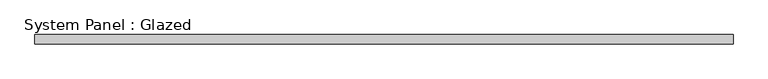
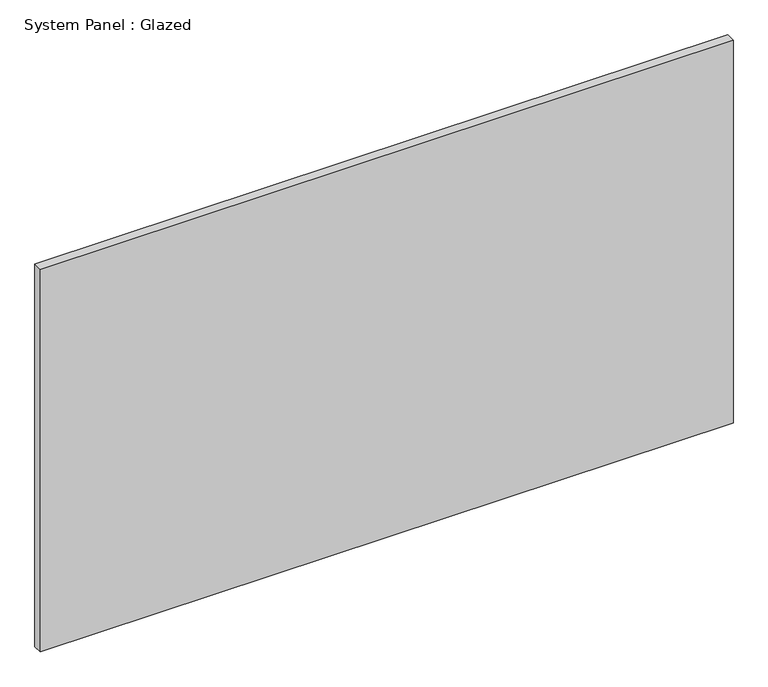
"""IFC4 building model written with IfcOpenShell, lengths in millimetres: plate geometry, System Panel : Glazed."""

from ifc_helpers import new_model, si_unit, origin, origin_with_axes, place, context, project, spatial, polyline, outline, extrude, source, transform, mapped, element, save


def system_panel_glazed_6149afab(model_context):
    return source(origin(), model_context, "Body", "SweptSolid", [
        extrude(outline(polyline([(913.4936087, 24.5), (-913.4936087, 24.5), (-913.4936087, 49.5), (913.4936087, 49.5), (913.4936087, 24.5)])), origin_with_axes(), (0.0, 0.0, 1.0), 1067.1518548),
    ])


if __name__ == "__main__":
    model = new_model("IFC4")
    model_context = context("Model", 3, world=origin())
    ifc_project = project(units=[si_unit("LENGTHUNIT", "METRE", prefix="MILLI")], contexts=[model_context])
    site = spatial("IfcSite", under=ifc_project)
    building = spatial("IfcBuilding", under=site)
    placement = place(None, origin())
    system_panel_glazed_shape = system_panel_glazed_6149afab(model_context)
    element("IfcPlate", 1, ObjectType="System Panel : Glazed", at=placement, inside=building, context=model_context, shape_type="MappedRepresentation", body=[
        mapped(system_panel_glazed_shape, transform((0.0, 0.0, 0.0), x_axis=(1.0, 0.0, 0.0), y_axis=(0.0, 1.0, 0.0), z_axis=(0.0, 0.0, 1.0))),
    ])
    save(model, "model.ifc")

# Revit data of these elements
# Type "System Panel : Glazed"
#   Keynote = "H11"
#   Construction Type Id = "GSP4R"
#   Analytic Construction = "1/8 in Pilkington single glazing"
#   Visual Light Transmittance = 0.9
#   Solar Heat Gain Coefficient = 0.86
#   Heat Transfer Coefficient (U) = 6.7069 W/(m²·K)
#   Define Thermal Properties by = 1
# Element 1 (IfcPlate, "System Panel : Glazed")
#   Materials on its faces: "Glass"
# Materials
#   "Glass": class "Glass", colour RGB 0 128 192, transparency 0.9, Description = "Soda Lime Glass", Cost = 0
